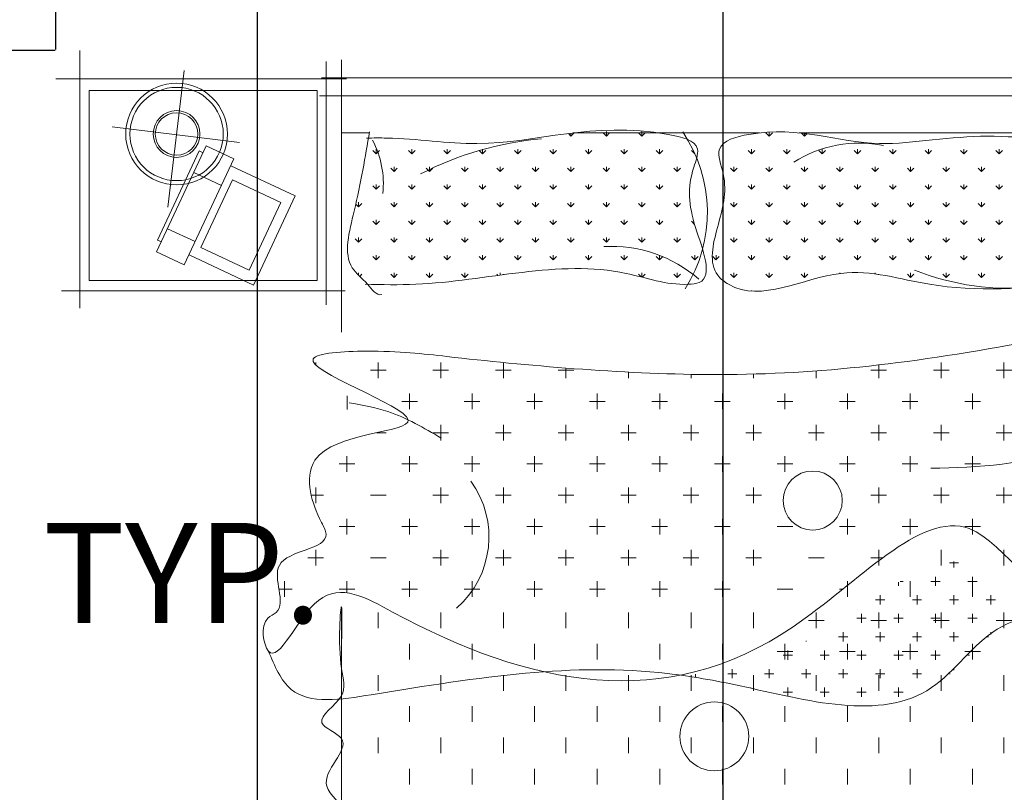
# Model space of a CAD drawing. Units: inches. Extents: x -438 to 102, y -60 to 1091.
# Tile 12 of 20: x -322 to -243, y 961 to 1022. Entities that reach past the tile are written whole.
import ezdxf

# ---------------------------------------------------------------- set-up
doc = ezdxf.new("R2010")
doc.units = ezdxf.units.IN
doc.header["$MEASUREMENT"] = 0
doc.layers.add('A-ANNO-DIMS', color=217, linetype='Continuous', lineweight=18, true_color=0x93278f)
doc.layers.add('Furniture', color=7, linetype='Continuous', lineweight=15)
doc.styles.get("Standard").update_dxf_attribs({"font": 'arial.ttf'})
doc.dimstyles.get("Standard").update_dxf_attribs({"dimtxt": 8, "dimasz": 0.18, "dimexe": 0.18, "dimexo": 0.0625, "dimgap": 0.09, "dimtad": 0, "dimtih": 1, "dimtoh": 1, "dimdec": 4, "dimzin": 0, "dimdsep": 46, "dimlunit": 3, "dimtxsty": 'Standard', "dimcen": 0.09, "dimadec": 0, "dimazin": 0, "dimtfac": 1, "dimtdec": 4, "dimtofl": 0, "dimtmove": 0, "dimatfit": 3, "dimfxl": 1, "dimtolj": 1, "dimtzin": 0, "dimarcsym": 0})

# ---------------------------------------------------------------- blocks, each defined once
blk = doc.blocks.new('BED-DOUBLE-WITH-NIGHTSTANDS')
for p, q in [((-50.059, 0.003), (-50.059, -20.597)), ((-29.157, -22.53), (-29.157, -0.743)), ((-30.374, -20.327), (-30.374, -0.897)), ((-28.759, -2.28), (-51.984, -2.28)), ((-41.716, -1.597), (-43.046, -12.532)), ((-30.745, -2.188), (29.898, -2.188)), ((-31.095, -3.205), (-49.317, -3.205)), ((-49.317, -3.205), (-49.317, -18.39)), ((-31.095, -18.39), (-31.095, -3.205)), ((30.685, -3.641), (-30.922, -3.641)), ((-37.317, -7.352), (-47.474, -6.101)), ((-26.928, -6.593), (-29.157, -6.593)), ((-10.816, -6.85), (-11.024, -6.642)), ((-10.816, -6.85), (-10.551, -6.585)), ((-10.816, -6.851), (-10.816, -6.616)), ((4.241, -6.593), (-10.627, -6.593)), ((-7.988, -6.85), (-8.253, -6.585)), ((-7.988, -6.85), (-7.723, -6.585)), ((-7.987, -6.851), (-7.987, -6.476)), ((-5.159, -6.85), (-5.425, -6.585)), ((-5.159, -6.851), (-5.159, -6.476)), ((-5.159, -6.85), (-4.894, -6.585)), ((5.018, -6.85), (4.753, -6.585)), ((5.018, -6.851), (5.018, -6.53)), ((5.018, -6.85), (5.283, -6.585)), ((29.898, -6.593), (7.41, -6.593)), ((7.846, -6.85), (7.61, -6.614)), ((7.846, -6.85), (8.033, -6.663)), ((7.847, -6.851), (7.847, -6.641)), ((-43.928, -16.114), (-39.959, -7.633)), ((-39.959, -7.633), (-37.75, -8.667)), ((-40.527, -8.034), (-43.863, -15.161)), ((-40.215, -8.18), (-40.527, -8.034)), ((-26.373, -8.265), (-26.638, -8)), ((-26.373, -8.265), (-26.107, -8)), ((-26.372, -8.265), (-26.372, -7.89)), ((-23.544, -8.265), (-23.809, -8)), ((-23.544, -8.265), (-23.544, -7.89)), ((-23.544, -8.265), (-23.279, -8)), ((-20.716, -8.265), (-20.981, -8)), ((-20.716, -8.265), (-20.451, -8)), ((-20.715, -8.265), (-20.715, -7.89)), ((-17.887, -8.265), (-18.152, -8)), ((-17.887, -8.265), (-17.887, -7.89)), ((-17.887, -8.265), (-17.622, -8)), ((-15.059, -8.265), (-15.324, -8)), ((-15.059, -8.265), (-14.794, -8)), ((-15.058, -8.265), (-15.058, -7.89)), ((-12.23, -8.265), (-12.496, -8)), ((-12.23, -8.265), (-12.23, -7.89)), ((-12.23, -8.265), (-11.965, -8)), ((-9.402, -8.265), (-9.667, -8)), ((-9.402, -8.265), (-9.402, -7.89)), ((-9.402, -8.265), (-9.137, -8)), ((-6.574, -8.265), (-6.839, -8)), ((-6.574, -8.265), (-6.308, -8)), ((-6.573, -8.265), (-6.573, -7.89)), ((-3.745, -8.265), (-4.01, -8)), ((-3.745, -8.265), (-3.745, -7.89)), ((-3.745, -8.265), (-3.48, -8)), ((-0.917, -8.265), (-1.182, -8)), ((-0.917, -8.265), (-0.915, -8.262)), ((-0.916, -8.265), (-0.916, -8.258)), ((1.02, -8.021), (1.041, -8)), ((3.604, -8.265), (3.339, -8)), ((3.604, -8.265), (3.604, -7.89)), ((3.604, -8.265), (3.869, -8)), ((6.432, -8.265), (6.167, -8)), ((6.432, -8.265), (6.697, -8)), ((6.433, -8.265), (6.433, -7.89)), ((9.261, -8.265), (8.996, -8)), ((9.261, -8.265), (9.261, -7.89)), ((9.261, -8.265), (9.526, -8)), ((12.089, -8.265), (11.824, -8)), ((12.089, -8.265), (12.089, -7.89)), ((12.089, -8.265), (12.354, -8)), ((14.918, -8.265), (14.652, -8)), ((14.918, -8.265), (14.918, -7.89)), ((14.918, -8.265), (15.183, -8)), ((17.746, -8.265), (17.481, -8)), ((17.746, -8.265), (17.746, -7.89)), ((17.746, -8.265), (18.011, -8)), ((20.574, -8.265), (20.309, -8)), ((20.574, -8.265), (20.84, -8)), ((20.575, -8.265), (20.575, -7.89)), ((23.403, -8.265), (23.138, -8)), ((23.403, -8.265), (23.403, -7.89)), ((23.403, -8.265), (23.668, -8)), ((-37.75, -8.667), (-41.72, -17.147)), ((-32.845, -11.63), (-38.006, -9.214)), ((-24.958, -9.679), (-25.224, -9.414)), ((-24.958, -9.679), (-24.958, -9.304)), ((-24.958, -9.679), (-24.693, -9.414)), ((-22.13, -9.679), (-22.395, -9.414)), ((-22.13, -9.679), (-22.13, -9.304)), ((-22.13, -9.679), (-21.865, -9.414)), ((-19.302, -9.679), (-19.567, -9.414)), ((-19.302, -9.679), (-19.036, -9.414)), ((-19.301, -9.679), (-19.301, -9.304)), ((-16.473, -9.679), (-16.738, -9.414)), ((-16.473, -9.679), (-16.473, -9.304)), ((-16.473, -9.679), (-16.208, -9.414)), ((-13.645, -9.679), (-13.91, -9.414)), ((-13.645, -9.679), (-13.38, -9.414)), ((-13.644, -9.679), (-13.644, -9.304)), ((-10.816, -9.679), (-11.081, -9.414)), ((-10.816, -9.679), (-10.816, -9.304)), ((-10.816, -9.679), (-10.551, -9.414)), ((-7.988, -9.679), (-8.253, -9.414)), ((-7.988, -9.679), (-7.723, -9.414)), ((-7.987, -9.679), (-7.987, -9.304)), ((-5.159, -9.679), (-5.425, -9.414)), ((-5.159, -9.679), (-5.159, -9.304)), ((-5.159, -9.679), (-4.894, -9.414)), ((-2.331, -9.679), (-2.596, -9.414)), ((-2.331, -9.679), (-2.331, -9.304)), ((-2.331, -9.679), (-2.066, -9.414)), ((2.19, -9.679), (1.924, -9.414)), ((2.19, -9.679), (2.19, -9.304)), ((2.19, -9.679), (2.455, -9.414)), ((5.018, -9.679), (4.753, -9.414)), ((5.018, -9.679), (5.018, -9.304)), ((5.018, -9.679), (5.283, -9.414)), ((7.846, -9.679), (7.581, -9.414)), ((7.846, -9.679), (8.112, -9.414)), ((7.847, -9.679), (7.847, -9.304)), ((10.675, -9.679), (10.41, -9.414)), ((10.675, -9.679), (10.675, -9.304)), ((10.675, -9.679), (10.94, -9.414)), ((13.503, -9.679), (13.238, -9.414)), ((13.503, -9.679), (13.768, -9.414)), ((13.504, -9.679), (13.504, -9.304)), ((16.332, -9.679), (16.067, -9.414)), ((16.332, -9.679), (16.332, -9.304)), ((16.332, -9.679), (16.597, -9.414)), ((19.16, -9.679), (18.895, -9.414)), ((19.16, -9.679), (19.425, -9.414)), ((19.161, -9.679), (19.161, -9.304)), ((21.989, -9.679), (21.723, -9.414)), ((21.989, -9.679), (21.989, -9.304)), ((21.989, -9.679), (22.254, -9.414)), ((-38.742, -10.787), (-40.951, -9.753)), ((-37.855, -10.358), (-40.387, -15.767)), ((-34.001, -12.162), (-37.855, -10.358)), ((-26.373, -11.093), (-26.638, -10.828)), ((-26.373, -11.093), (-26.107, -10.828)), ((-26.372, -11.093), (-26.372, -10.718)), ((-23.544, -11.093), (-23.809, -10.828)), ((-23.544, -11.093), (-23.544, -10.718)), ((-23.544, -11.093), (-23.279, -10.828)), ((-20.716, -11.093), (-20.981, -10.828)), ((-20.716, -11.093), (-20.451, -10.828)), ((-20.715, -11.093), (-20.715, -10.718)), ((-17.887, -11.093), (-18.152, -10.828)), ((-17.887, -11.093), (-17.887, -10.718)), ((-17.887, -11.093), (-17.622, -10.828)), ((-15.059, -11.093), (-15.324, -10.828)), ((-15.059, -11.093), (-14.794, -10.828)), ((-15.058, -11.093), (-15.058, -10.718)), ((-12.23, -11.093), (-12.496, -10.828)), ((-12.23, -11.093), (-12.23, -10.718)), ((-12.23, -11.093), (-11.965, -10.828)), ((-9.402, -11.093), (-9.667, -10.828)), ((-9.402, -11.093), (-9.402, -10.718)), ((-9.402, -11.093), (-9.137, -10.828)), ((-6.574, -11.093), (-6.839, -10.828)), ((-6.574, -11.093), (-6.308, -10.828)), ((-6.573, -11.093), (-6.573, -10.718)), ((-3.745, -11.093), (-4.01, -10.828)), ((-3.745, -11.093), (-3.745, -10.718)), ((-3.745, -11.093), (-3.48, -10.828)), ((3.604, -11.093), (3.339, -10.828)), ((3.604, -11.093), (3.604, -10.718)), ((3.604, -11.093), (3.869, -10.828)), ((6.432, -11.093), (6.167, -10.828)), ((6.432, -11.093), (6.697, -10.828)), ((6.433, -11.093), (6.433, -10.718)), ((9.261, -11.093), (8.996, -10.828)), ((9.261, -11.093), (9.261, -10.718)), ((9.261, -11.093), (9.526, -10.828)), ((12.089, -11.093), (11.824, -10.828)), ((12.089, -11.093), (12.089, -10.718)), ((12.089, -11.093), (12.354, -10.828)), ((14.918, -11.093), (14.652, -10.828)), ((14.918, -11.093), (14.918, -10.718)), ((14.918, -11.093), (15.183, -10.828)), ((17.746, -11.093), (17.481, -10.828)), ((17.746, -11.093), (17.746, -10.718)), ((17.746, -11.093), (18.011, -10.828)), ((20.574, -11.093), (20.309, -10.828)), ((20.574, -11.093), (20.84, -10.828)), ((20.575, -11.093), (20.575, -10.718)), ((23.403, -11.093), (23.138, -10.828)), ((23.403, -11.093), (23.403, -10.718)), ((23.403, -11.093), (23.668, -10.828)), ((-36.181, -18.757), (-32.845, -11.63)), ((-36.532, -17.571), (-34.001, -12.162)), ((-27.787, -12.507), (-28.013, -12.281)), ((-27.787, -12.507), (-27.522, -12.242)), ((-27.786, -12.508), (-27.786, -12.133)), ((-24.958, -12.507), (-25.224, -12.242)), ((-24.958, -12.508), (-24.958, -12.133)), ((-24.958, -12.507), (-24.693, -12.242)), ((-22.13, -12.507), (-22.395, -12.242)), ((-22.13, -12.508), (-22.13, -12.133)), ((-22.13, -12.507), (-21.865, -12.242)), ((-19.302, -12.507), (-19.567, -12.242)), ((-19.302, -12.507), (-19.036, -12.242)), ((-19.301, -12.508), (-19.301, -12.133)), ((-16.473, -12.507), (-16.738, -12.242)), ((-16.473, -12.508), (-16.473, -12.133)), ((-16.473, -12.507), (-16.208, -12.242)), ((-13.645, -12.507), (-13.91, -12.242)), ((-13.645, -12.507), (-13.38, -12.242)), ((-13.644, -12.508), (-13.644, -12.133)), ((-10.816, -12.507), (-11.081, -12.242)), ((-10.816, -12.508), (-10.816, -12.133)), ((-10.816, -12.507), (-10.551, -12.242)), ((-7.988, -12.507), (-8.253, -12.242)), ((-7.988, -12.507), (-7.723, -12.242)), ((-7.987, -12.508), (-7.987, -12.133)), ((-5.159, -12.507), (-5.425, -12.242)), ((-5.159, -12.508), (-5.159, -12.133)), ((-5.159, -12.507), (-4.894, -12.242)), ((-2.331, -12.507), (-2.596, -12.242)), ((-2.331, -12.508), (-2.331, -12.133)), ((-2.331, -12.507), (-2.066, -12.242)), ((2.19, -12.507), (1.924, -12.242)), ((2.19, -12.508), (2.19, -12.133)), ((2.19, -12.507), (2.455, -12.242)), ((5.018, -12.507), (4.753, -12.242)), ((5.018, -12.508), (5.018, -12.133)), ((5.018, -12.507), (5.283, -12.242)), ((7.846, -12.507), (7.581, -12.242)), ((7.846, -12.507), (8.112, -12.242)), ((7.847, -12.508), (7.847, -12.133)), ((10.675, -12.507), (10.41, -12.242)), ((10.675, -12.508), (10.675, -12.133)), ((10.675, -12.507), (10.94, -12.242)), ((13.503, -12.507), (13.238, -12.242)), ((13.503, -12.507), (13.768, -12.242)), ((13.504, -12.508), (13.504, -12.133)), ((16.332, -12.507), (16.067, -12.242)), ((16.332, -12.508), (16.332, -12.133)), ((16.332, -12.507), (16.597, -12.242)), ((19.16, -12.507), (18.895, -12.242)), ((19.16, -12.507), (19.425, -12.242)), ((19.161, -12.508), (19.161, -12.133)), ((21.989, -12.507), (21.723, -12.242)), ((21.989, -12.508), (21.989, -12.133)), ((21.989, -12.507), (22.254, -12.242)), ((-26.373, -13.922), (-26.638, -13.656)), ((-26.373, -13.922), (-26.107, -13.656)), ((-26.372, -13.922), (-26.372, -13.547)), ((-23.544, -13.922), (-23.809, -13.656)), ((-23.544, -13.922), (-23.544, -13.547)), ((-23.544, -13.922), (-23.279, -13.656)), ((-20.716, -13.922), (-20.981, -13.656)), ((-20.716, -13.922), (-20.451, -13.656)), ((-20.715, -13.922), (-20.715, -13.547)), ((-17.887, -13.922), (-18.152, -13.656)), ((-17.887, -13.922), (-17.887, -13.547)), ((-17.887, -13.922), (-17.622, -13.656)), ((-15.059, -13.922), (-15.324, -13.656)), ((-15.059, -13.922), (-14.794, -13.656)), ((-15.058, -13.922), (-15.058, -13.547)), ((-12.23, -13.922), (-12.496, -13.656)), ((-12.23, -13.922), (-12.23, -13.547)), ((-12.23, -13.922), (-11.965, -13.656)), ((-9.402, -13.922), (-9.667, -13.656)), ((-9.402, -13.922), (-9.402, -13.547)), ((-9.402, -13.922), (-9.137, -13.656)), ((-6.574, -13.922), (-6.839, -13.656)), ((-6.574, -13.922), (-6.308, -13.656)), ((-6.573, -13.922), (-6.573, -13.547)), ((-3.745, -13.922), (-4.01, -13.656)), ((-3.745, -13.922), (-3.745, -13.547)), ((-3.745, -13.922), (-3.48, -13.656)), ((-0.933, -13.906), (-1.182, -13.656)), ((1.022, -13.675), (1.041, -13.656)), ((3.604, -13.922), (3.339, -13.656)), ((3.604, -13.922), (3.604, -13.547)), ((3.604, -13.922), (3.869, -13.656)), ((6.432, -13.922), (6.167, -13.656)), ((6.432, -13.922), (6.697, -13.656)), ((6.433, -13.922), (6.433, -13.547)), ((9.261, -13.922), (8.996, -13.656)), ((9.261, -13.922), (9.261, -13.547)), ((9.261, -13.922), (9.526, -13.656)), ((12.089, -13.922), (11.824, -13.656)), ((12.089, -13.922), (12.089, -13.547)), ((12.089, -13.922), (12.354, -13.656)), ((14.918, -13.922), (14.652, -13.656)), ((14.918, -13.922), (14.918, -13.547)), ((14.918, -13.922), (15.183, -13.656)), ((17.746, -13.922), (17.481, -13.656)), ((17.746, -13.922), (17.746, -13.547)), ((17.746, -13.922), (18.011, -13.656)), ((20.574, -13.922), (20.309, -13.656)), ((20.574, -13.922), (20.84, -13.656)), ((20.575, -13.922), (20.575, -13.547)), ((23.403, -13.922), (23.138, -13.656)), ((23.403, -13.922), (23.403, -13.547)), ((23.403, -13.922), (23.668, -13.656)), ((-40.849, -15.287), (-43.058, -14.253)), ((-43.863, -15.161), (-43.551, -15.307)), ((-27.787, -15.336), (-28.052, -15.071)), ((-27.787, -15.336), (-27.522, -15.071)), ((-27.786, -15.336), (-27.786, -14.961)), ((-24.958, -15.336), (-25.224, -15.071)), ((-24.958, -15.336), (-24.958, -14.961)), ((-24.958, -15.336), (-24.693, -15.071)), ((-22.13, -15.336), (-22.395, -15.071)), ((-22.13, -15.336), (-22.13, -14.961)), ((-22.13, -15.336), (-21.865, -15.071)), ((-19.302, -15.336), (-19.567, -15.071)), ((-19.302, -15.336), (-19.036, -15.071)), ((-19.301, -15.336), (-19.301, -14.961)), ((-16.473, -15.336), (-16.738, -15.071)), ((-16.473, -15.336), (-16.473, -14.961)), ((-16.473, -15.336), (-16.208, -15.071)), ((-13.645, -15.336), (-13.91, -15.071)), ((-13.645, -15.336), (-13.38, -15.071)), ((-13.644, -15.336), (-13.644, -14.961)), ((-10.816, -15.336), (-11.081, -15.071)), ((-10.816, -15.336), (-10.816, -14.961)), ((-10.816, -15.336), (-10.551, -15.071)), ((-7.988, -15.336), (-8.253, -15.071)), ((-7.988, -15.336), (-7.723, -15.071)), ((-7.987, -15.336), (-7.987, -14.961)), ((-5.159, -15.336), (-5.425, -15.071)), ((-5.159, -15.336), (-5.159, -14.961)), ((-5.159, -15.336), (-4.894, -15.071)), ((-2.331, -15.336), (-2.596, -15.071)), ((-2.331, -15.336), (-2.331, -14.961)), ((-2.331, -15.336), (-2.066, -15.071)), ((2.19, -15.336), (1.924, -15.071)), ((2.19, -15.336), (2.19, -14.961)), ((2.19, -15.336), (2.455, -15.071)), ((5.018, -15.336), (4.753, -15.071)), ((5.018, -15.336), (5.018, -14.961)), ((5.018, -15.336), (5.283, -15.071)), ((7.846, -15.336), (7.581, -15.071)), ((7.846, -15.336), (8.112, -15.071)), ((7.847, -15.336), (7.847, -14.961)), ((10.675, -15.336), (10.41, -15.071)), ((10.675, -15.336), (10.675, -14.961)), ((10.675, -15.336), (10.94, -15.071)), ((13.503, -15.336), (13.238, -15.071)), ((13.503, -15.336), (13.768, -15.071)), ((13.504, -15.336), (13.504, -14.961)), ((16.332, -15.336), (16.067, -15.071)), ((16.332, -15.336), (16.332, -14.961)), ((16.332, -15.336), (16.597, -15.071)), ((19.16, -15.336), (18.895, -15.071)), ((19.16, -15.336), (19.425, -15.071)), ((19.161, -15.336), (19.161, -14.961)), ((21.989, -15.336), (21.723, -15.071)), ((21.989, -15.336), (21.989, -14.961)), ((21.989, -15.336), (22.254, -15.071)), ((-41.72, -17.147), (-43.928, -16.114)), ((-41.342, -16.341), (-36.181, -18.757)), ((-40.387, -15.767), (-36.532, -17.571)), ((-26.373, -16.75), (-26.638, -16.485)), ((-26.373, -16.75), (-26.107, -16.485)), ((-26.372, -16.75), (-26.372, -16.375)), ((-23.544, -16.75), (-23.809, -16.485)), ((-23.544, -16.75), (-23.544, -16.375)), ((-23.544, -16.75), (-23.279, -16.485)), ((-20.716, -16.75), (-20.981, -16.485)), ((-20.716, -16.75), (-20.451, -16.485)), ((-20.715, -16.75), (-20.715, -16.375)), ((-17.887, -16.75), (-18.152, -16.485)), ((-17.887, -16.75), (-17.887, -16.375)), ((-17.887, -16.75), (-17.622, -16.485)), ((-15.059, -16.75), (-15.324, -16.485)), ((-15.059, -16.75), (-14.794, -16.485)), ((-15.058, -16.75), (-15.058, -16.375)), ((-12.23, -16.75), (-12.496, -16.485)), ((-12.23, -16.75), (-12.23, -16.375)), ((-12.23, -16.75), (-11.965, -16.485)), ((-9.402, -16.75), (-9.667, -16.485)), ((-9.402, -16.75), (-9.402, -16.375)), ((-9.402, -16.75), (-9.137, -16.485)), ((-6.574, -16.75), (-6.839, -16.485)), ((-6.574, -16.75), (-6.308, -16.485)), ((-6.573, -16.75), (-6.573, -16.375)), ((-3.745, -16.75), (-4.01, -16.485)), ((-3.745, -16.75), (-3.745, -16.375)), ((-3.745, -16.75), (-3.48, -16.485)), ((-0.917, -16.75), (-1.182, -16.485)), ((-0.917, -16.75), (-0.652, -16.485)), ((-0.916, -16.75), (-0.916, -16.375)), ((0.775, -16.75), (0.51, -16.485)), ((0.775, -16.75), (1.041, -16.485)), ((0.776, -16.75), (0.776, -16.375)), ((3.604, -16.75), (3.339, -16.485)), ((3.604, -16.75), (3.604, -16.375)), ((3.604, -16.75), (3.869, -16.485)), ((6.432, -16.75), (6.167, -16.485)), ((6.432, -16.75), (6.697, -16.485)), ((6.433, -16.75), (6.433, -16.375)), ((9.261, -16.75), (8.996, -16.485)), ((9.261, -16.75), (9.261, -16.375)), ((9.261, -16.75), (9.526, -16.485)), ((12.089, -16.75), (11.824, -16.485)), ((12.089, -16.75), (12.089, -16.375)), ((12.089, -16.75), (12.354, -16.485)), ((14.918, -16.75), (14.652, -16.485)), ((14.918, -16.75), (14.918, -16.375)), ((14.918, -16.75), (15.183, -16.485)), ((17.746, -16.75), (17.481, -16.485)), ((17.746, -16.75), (17.746, -16.375)), ((17.746, -16.75), (18.011, -16.485)), ((20.574, -16.75), (20.309, -16.485)), ((20.574, -16.75), (20.84, -16.485)), ((20.575, -16.75), (20.575, -16.375)), ((23.403, -16.75), (23.138, -16.485)), ((23.403, -16.75), (23.403, -16.375)), ((23.403, -16.75), (23.668, -16.485)), ((-27.786, -17.973), (-27.786, -17.79)), ((-27.69, -18.067), (-27.522, -17.899)), ((-24.958, -18.164), (-25.224, -17.899)), ((-24.958, -18.165), (-24.958, -17.79)), ((-24.958, -18.164), (-24.693, -17.899)), ((-22.13, -18.164), (-22.395, -17.899)), ((-22.13, -18.165), (-22.13, -17.79)), ((-22.13, -18.164), (-21.865, -17.899)), ((-19.302, -18.164), (-19.567, -17.899)), ((-19.302, -18.164), (-19.036, -17.899)), ((-19.301, -18.165), (-19.301, -17.79)), ((-16.65, -17.987), (-16.738, -17.899)), ((-16.473, -17.964), (-16.473, -17.79)), ((-16.242, -17.933), (-16.208, -17.899)), ((-5.211, -18.113), (-5.425, -17.899)), ((-5.159, -18.126), (-5.159, -17.79)), ((-5.129, -18.134), (-4.894, -17.899)), ((-2.331, -18.164), (-2.596, -17.899)), ((-2.331, -18.165), (-2.331, -17.79)), ((-2.331, -18.164), (-2.066, -17.899)), ((2.19, -18.164), (1.924, -17.899)), ((2.19, -18.165), (2.19, -17.79)), ((2.19, -18.164), (2.455, -17.899)), ((5.018, -18.164), (4.753, -17.899)), ((5.018, -18.165), (5.018, -17.79)), ((5.018, -18.164), (5.283, -17.899)), ((7.846, -18.164), (7.581, -17.899)), ((7.846, -18.164), (8.112, -17.899)), ((7.847, -18.165), (7.847, -17.79)), ((10.675, -17.833), (10.675, -17.79)), ((13.504, -17.877), (13.504, -17.79)), ((13.756, -17.912), (13.768, -17.899)), ((16.332, -18.164), (16.067, -17.899)), ((16.332, -18.165), (16.332, -17.79)), ((16.332, -18.164), (16.597, -17.899)), ((19.16, -18.164), (18.895, -17.899)), ((19.16, -18.164), (19.425, -17.899)), ((19.161, -18.165), (19.161, -17.79)), ((21.989, -18.164), (21.723, -17.899)), ((21.989, -18.165), (21.989, -17.79)), ((21.989, -18.164), (22.254, -17.899)), ((-49.317, -18.39), (-31.095, -18.39)), ((-51.534, -19.209), (-28.849, -19.209)), ((3.604, -19.237), (3.604, -19.204)), ((-31.218, -25.145), (-31.218, -24.94)), ((-26.218, -26.19), (-26.218, -24.94)), ((-21.218, -26.19), (-21.218, -24.94)), ((-16.218, -26.19), (-16.218, -24.951)), ((13.782, -26.19), (13.782, -25.145)), ((18.782, -26.19), (18.782, -24.94)), ((23.782, -26.19), (23.782, -24.94)), ((-30.593, -25.565), (-30.673, -25.565)), ((-25.593, -25.565), (-26.843, -25.565)), ((-20.593, -25.565), (-21.843, -25.565)), ((-15.593, -25.565), (-16.843, -25.565)), ((-10.593, -25.565), (-11.843, -25.565)), ((-11.218, -26.19), (-11.218, -25.392)), ((-6.218, -26.19), (-6.218, -25.718)), ((-1.218, -26.19), (-1.218, -25.896)), ((3.782, -26.19), (3.782, -25.874)), ((8.782, -26.19), (8.782, -25.623)), ((14.407, -25.565), (13.157, -25.565)), ((19.407, -25.565), (18.157, -25.565)), ((24.407, -25.565), (23.157, -25.565)), ((-23.718, -28.69), (-23.718, -27.44)), ((-18.718, -28.69), (-18.718, -27.44)), ((-13.718, -28.69), (-13.718, -27.44)), ((-8.718, -28.69), (-8.718, -27.44)), ((-3.718, -28.69), (-3.718, -27.44)), ((1.282, -28.69), (1.282, -27.44)), ((6.282, -28.69), (6.282, -27.44)), ((11.282, -28.69), (11.282, -27.44)), ((16.282, -28.69), (16.282, -27.44)), ((21.282, -28.69), (21.282, -27.44)), ((-28.711, -28.721), (-28.711, -27.603)), ((-23.093, -28.065), (-24.343, -28.065)), ((-18.093, -28.065), (-19.343, -28.065)), ((-13.093, -28.065), (-14.343, -28.065)), ((-8.093, -28.065), (-9.343, -28.065)), ((-3.093, -28.065), (-4.343, -28.065)), ((1.907, -28.065), (0.657, -28.065)), ((6.907, -28.065), (5.657, -28.065)), ((11.907, -28.065), (10.657, -28.065)), ((16.907, -28.065), (15.657, -28.065)), ((21.907, -28.065), (20.657, -28.065)), ((-25.593, -30.565), (-26.366, -30.565)), ((-20.593, -30.565), (-21.843, -30.565)), ((-21.218, -31.19), (-21.218, -29.94)), ((-15.593, -30.565), (-16.843, -30.565)), ((-16.218, -31.19), (-16.218, -29.94)), ((-10.593, -30.565), (-11.843, -30.565)), ((-11.218, -31.19), (-11.218, -29.94)), ((-5.593, -30.565), (-6.843, -30.565)), ((-6.218, -31.19), (-6.218, -29.94)), ((-0.593, -30.565), (-1.843, -30.565)), ((-1.218, -31.19), (-1.218, -29.94)), ((4.407, -30.565), (3.157, -30.565)), ((3.782, -31.19), (3.782, -29.94)), ((9.407, -30.565), (8.157, -30.565)), ((8.782, -31.19), (8.782, -29.94)), ((14.407, -30.565), (13.157, -30.565)), ((13.782, -31.19), (13.782, -29.94)), ((19.407, -30.565), (18.157, -30.565)), ((18.782, -31.19), (18.782, -29.94)), ((24.407, -30.565), (23.157, -30.565)), ((23.782, -31.19), (23.782, -29.94)), ((-28.718, -33.69), (-28.718, -32.44)), ((-23.718, -33.69), (-23.718, -32.44)), ((-18.718, -33.69), (-18.718, -32.44)), ((-13.718, -33.69), (-13.718, -32.44)), ((-8.718, -33.69), (-8.718, -32.44)), ((-3.718, -33.69), (-3.718, -32.44)), ((1.282, -33.69), (1.282, -32.44)), ((6.282, -33.69), (6.282, -32.44)), ((11.282, -33.69), (11.282, -32.44)), ((16.282, -33.69), (16.282, -32.44)), ((21.282, -33.69), (21.282, -32.44)), ((-28.093, -33.065), (-29.343, -33.065)), ((-23.093, -33.065), (-24.343, -33.065)), ((-18.093, -33.065), (-19.343, -33.065)), ((-13.093, -33.065), (-14.343, -33.065)), ((-8.093, -33.065), (-9.343, -33.065)), ((-3.093, -33.065), (-4.343, -33.065)), ((1.907, -33.065), (0.657, -33.065)), ((6.907, -33.065), (5.657, -33.065)), ((11.907, -33.065), (10.657, -33.065)), ((16.907, -33.065), (15.657, -33.065)), ((21.907, -33.065), (20.657, -33.065)), ((-31.218, -36.19), (-31.218, -34.94)), ((-21.218, -36.19), (-21.218, -34.94)), ((-16.218, -36.19), (-16.218, -34.94)), ((-11.218, -36.19), (-11.218, -34.94)), ((-6.218, -36.19), (-6.218, -34.94)), ((-1.218, -36.19), (-1.218, -34.94)), ((3.782, -36.19), (3.782, -34.94)), ((13.782, -36.19), (13.782, -34.94)), ((18.782, -36.19), (18.782, -34.94)), ((23.782, -36.19), (23.782, -34.94)), ((-30.593, -35.565), (-31.573, -35.565)), ((-25.593, -35.565), (-26.843, -35.565)), ((-20.593, -35.565), (-21.843, -35.565)), ((-15.593, -35.565), (-16.843, -35.565)), ((-10.593, -35.565), (-11.843, -35.565)), ((-5.593, -35.565), (-6.843, -35.565)), ((-0.593, -35.565), (-1.843, -35.565)), ((4.407, -35.565), (3.157, -35.565)), ((14.407, -35.565), (13.157, -35.565)), ((19.407, -35.565), (18.157, -35.565)), ((24.407, -35.565), (23.157, -35.565)), ((-28.718, -38.69), (-28.718, -37.44)), ((-23.718, -38.69), (-23.718, -37.44)), ((-18.718, -38.69), (-18.718, -37.44)), ((-13.718, -38.69), (-13.718, -37.44)), ((-8.718, -38.69), (-8.718, -37.44)), ((-3.718, -38.69), (-3.718, -37.44)), ((1.282, -38.69), (1.282, -37.44)), ((11.282, -38.69), (11.282, -37.44)), ((16.282, -38.69), (16.282, -37.44)), ((21.282, -38.69), (21.282, -37.44)), ((-28.093, -38.065), (-29.343, -38.065)), ((-23.093, -38.065), (-24.343, -38.065)), ((-18.093, -38.065), (-19.343, -38.065)), ((-13.093, -38.065), (-14.343, -38.065)), ((-8.093, -38.065), (-9.343, -38.065)), ((-3.093, -38.065), (-4.343, -38.065)), ((1.907, -38.065), (0.657, -38.065)), ((6.907, -38.065), (5.657, -38.065)), ((11.907, -38.065), (10.657, -38.065)), ((16.907, -38.065), (15.657, -38.065)), ((21.907, -38.065), (20.657, -38.065)), ((-31.218, -41.19), (-31.218, -39.94)), ((-21.218, -41.19), (-21.218, -39.94)), ((-16.218, -41.19), (-16.218, -39.94)), ((-11.218, -41.19), (-11.218, -39.94)), ((-6.218, -41.19), (-6.218, -39.94)), ((-1.218, -41.19), (-1.218, -39.94)), ((3.782, -41.19), (3.782, -39.94)), ((13.782, -41.19), (13.782, -39.94)), ((18.782, -41.19), (18.782, -39.94)), ((23.782, -41.19), (23.782, -39.94)), ((-30.593, -40.565), (-31.843, -40.565)), ((-25.593, -40.565), (-26.843, -40.565)), ((-20.593, -40.565), (-21.843, -40.565)), ((-15.593, -40.565), (-16.843, -40.565)), ((-10.593, -40.565), (-11.843, -40.565)), ((-5.593, -40.565), (-6.843, -40.565)), ((-0.593, -40.565), (-1.843, -40.565)), ((4.407, -40.565), (3.157, -40.565)), ((9.407, -40.565), (8.157, -40.565)), ((14.104, -40.565), (13.157, -40.565)), ((19.795, -41.341), (19.795, -40.863)), ((20.164, -40.972), (19.426, -40.972)), ((-33.718, -43.69), (-33.718, -42.44)), ((-28.718, -43.367), (-28.718, -42.44)), ((-23.718, -43.69), (-23.718, -42.44)), ((-18.718, -43.69), (-18.718, -42.44)), ((-13.718, -43.69), (-13.718, -42.44)), ((-8.718, -43.69), (-8.718, -42.44)), ((-3.718, -43.69), (-3.718, -42.44)), ((1.282, -43.69), (1.282, -42.44)), ((11.282, -43.69), (11.282, -42.44)), ((15.735, -42.448), (15.495, -42.448)), ((16.282, -43.69), (16.282, -42.44)), ((18.688, -42.448), (17.949, -42.448)), ((18.318, -42.817), (18.318, -42.079)), ((21.64, -42.448), (20.902, -42.448)), ((21.271, -42.817), (21.271, -42.079)), ((21.282, -43.69), (21.282, -42.44)), ((-33.093, -43.065), (-34.154, -43.065)), ((-28.093, -43.065), (-29.343, -43.065)), ((-23.093, -43.065), (-24.343, -43.065)), ((-18.093, -43.065), (-19.343, -43.065)), ((-13.093, -43.065), (-14.343, -43.065)), ((-8.093, -43.065), (-9.343, -43.065)), ((-3.093, -43.065), (-4.343, -43.065)), ((1.907, -43.065), (0.657, -43.065)), ((6.907, -43.065), (5.657, -43.065)), ((10.916, -43.065), (10.657, -43.065)), ((15.366, -42.817), (15.366, -42.522)), ((14.258, -43.924), (13.52, -43.924)), ((13.889, -44.294), (13.889, -43.555)), ((17.211, -43.924), (16.473, -43.924)), ((16.842, -44.294), (16.842, -43.555)), ((20.164, -43.924), (19.426, -43.924)), ((19.795, -44.294), (19.795, -43.555)), ((23.117, -43.924), (22.378, -43.924)), ((22.748, -44.294), (22.748, -43.555)), ((-29.157, -79.94), (-29.157, -44.493)), ((-26.218, -46.19), (-26.218, -44.94)), ((-21.218, -46.19), (-21.218, -44.94)), ((-16.218, -46.19), (-16.218, -44.94)), ((-11.218, -46.19), (-11.218, -44.94)), ((-6.218, -46.19), (-6.218, -44.94)), ((-1.218, -46.19), (-1.218, -44.94)), ((3.782, -46.19), (3.782, -44.94)), ((9.407, -45.565), (8.157, -45.565)), ((8.782, -46.19), (8.782, -44.94)), ((12.782, -45.401), (12.044, -45.401)), ((12.413, -45.77), (12.413, -45.032)), ((14.407, -45.565), (13.157, -45.565)), ((13.782, -46.19), (13.782, -44.94)), ((15.735, -45.401), (14.997, -45.401)), ((15.366, -45.77), (15.366, -45.032)), ((18.688, -45.401), (17.949, -45.401)), ((19.407, -45.565), (18.157, -45.565)), ((18.318, -45.77), (18.318, -45.032)), ((18.782, -46.19), (18.782, -44.94)), ((21.64, -45.401), (20.902, -45.401)), ((21.271, -45.77), (21.271, -45.032)), ((24.407, -45.565), (23.157, -45.565)), ((23.782, -46.19), (23.782, -44.94)), ((7.984, -47.246), (7.984, -47.199)), ((11.306, -46.877), (10.567, -46.877)), ((10.937, -47.246), (10.937, -46.508)), ((14.258, -46.877), (13.52, -46.877)), ((13.889, -47.246), (13.889, -46.508)), ((17.211, -46.877), (16.473, -46.877)), ((16.842, -47.246), (16.842, -46.508)), ((20.164, -46.877), (19.426, -46.877)), ((19.795, -47.246), (19.795, -46.508)), ((22.546, -46.877), (22.378, -46.877)), ((22.748, -46.697), (22.748, -46.508)), ((-23.718, -48.69), (-23.718, -47.44)), ((-18.718, -48.69), (-18.718, -47.44)), ((-13.718, -48.69), (-13.718, -47.44)), ((-8.718, -48.69), (-8.718, -47.44)), ((-3.718, -48.69), (-3.718, -47.44)), ((1.282, -48.69), (1.282, -47.44)), ((6.282, -48.69), (6.282, -47.44)), ((6.507, -48.723), (6.507, -47.984)), ((9.46, -48.723), (9.46, -47.984)), ((11.282, -48.69), (11.282, -47.44)), ((12.413, -48.723), (12.413, -47.984)), ((15.366, -48.723), (15.366, -47.984)), ((16.282, -48.69), (16.282, -47.44)), ((18.318, -48.723), (18.318, -47.984)), ((21.271, -48.106), (21.271, -47.984)), ((21.282, -48.69), (21.282, -47.44)), ((-34.327, -48.065), (-34.343, -48.065)), ((6.907, -48.065), (5.657, -48.065)), ((6.877, -48.354), (6.138, -48.354)), ((9.829, -48.354), (9.091, -48.354)), ((11.907, -48.065), (10.657, -48.065)), ((12.782, -48.354), (12.044, -48.354)), ((15.735, -48.354), (14.997, -48.354)), ((16.907, -48.065), (15.657, -48.065)), ((18.688, -48.354), (17.949, -48.354)), ((21.907, -48.065), (20.657, -48.065)), ((21.024, -48.354), (20.902, -48.354)), ((2.078, -50.199), (2.078, -49.461)), ((5.031, -50.199), (5.031, -49.461)), ((7.984, -50.199), (7.984, -49.461)), ((10.937, -50.199), (10.937, -49.461)), ((13.889, -50.199), (13.889, -49.461)), ((16.842, -50.199), (16.842, -49.461)), ((19.795, -49.55), (19.795, -49.461)), ((-26.218, -51.19), (-26.218, -49.94)), ((-21.218, -51.19), (-21.218, -49.94)), ((-16.218, -51.19), (-16.218, -49.94)), ((-11.218, -51.19), (-11.218, -49.94)), ((-6.218, -51.19), (-6.218, -49.94)), ((-1.218, -51.19), (-1.218, -49.94)), ((-0.874, -50.112), (-0.874, -49.874)), ((2.447, -49.83), (1.709, -49.83)), ((3.782, -51.19), (3.782, -49.94)), ((5.4, -49.83), (4.662, -49.83)), ((8.353, -49.83), (7.615, -49.83)), ((8.782, -51.19), (8.782, -49.94)), ((11.306, -49.83), (10.567, -49.83)), ((14.258, -49.83), (13.52, -49.83)), ((13.782, -51.19), (13.782, -49.94)), ((17.211, -49.83), (16.473, -49.83)), ((18.782, -51.19), (18.782, -49.94)), ((19.485, -49.83), (19.426, -49.83)), ((23.782, -51.19), (23.782, -49.94)), ((3.555, -50.987), (3.555, -50.937)), ((6.507, -51.614), (6.507, -50.937)), ((9.46, -51.675), (9.46, -50.937)), ((12.413, -51.675), (12.413, -50.937)), ((15.366, -51.675), (15.366, -50.937)), ((6.877, -51.306), (6.138, -51.306)), ((9.829, -51.306), (9.091, -51.306)), ((12.782, -51.306), (12.044, -51.306)), ((15.735, -51.306), (14.997, -51.306)), ((-23.718, -53.69), (-23.718, -52.44)), ((-18.718, -53.69), (-18.718, -52.44)), ((-13.718, -53.69), (-13.718, -52.44)), ((-8.718, -53.69), (-8.718, -52.44)), ((-3.718, -53.69), (-3.718, -52.44)), ((1.282, -53.69), (1.282, -52.44)), ((6.282, -53.69), (6.282, -52.44)), ((11.282, -53.69), (11.282, -52.44)), ((16.282, -53.69), (16.282, -52.44)), ((21.282, -53.69), (21.282, -52.44)), ((-26.218, -56.19), (-26.218, -54.94)), ((-21.218, -56.19), (-21.218, -54.94)), ((-16.218, -56.19), (-16.218, -54.94)), ((-11.218, -56.19), (-11.218, -54.94)), ((-6.218, -56.19), (-6.218, -54.94)), ((-1.218, -56.19), (-1.218, -54.94)), ((3.782, -56.19), (3.782, -54.94)), ((8.782, -56.19), (8.782, -54.94)), ((13.782, -56.19), (13.782, -54.94)), ((18.782, -56.19), (18.782, -54.94)), ((23.782, -56.19), (23.782, -54.94)), ((-23.718, -58.69), (-23.718, -57.44)), ((-18.718, -58.69), (-18.718, -57.44)), ((-13.718, -58.69), (-13.718, -57.44)), ((-8.718, -58.69), (-8.718, -57.44)), ((-3.718, -58.69), (-3.718, -57.44)), ((1.282, -58.69), (1.282, -57.44)), ((6.282, -58.69), (6.282, -57.44)), ((11.282, -58.69), (11.282, -57.44)), ((16.282, -58.69), (16.282, -57.44)), ((21.282, -58.69), (21.282, -57.44))]:
    blk.add_line(p, q)
for centre, radius in [((-42.334, -6.681), 4.065), ((-42.334, -6.681), 3.73), ((-42.334, -6.681), 1.87), ((-42.334, -6.681), 1.702), ((8.508, -35.984), 2.359), ((0.643, -54.842), 2.753)]:
    blk.add_circle(centre, radius)
for centre, radius, start, end in [((-10.895, -32.973), 26.004, 95.02643, 117.32994), ((-11.37, -12.946), 11.457, 327.75554, 34.13971), ((-33.344, -10.683), 7.534, 354.32477, 27.77276), ((12.254, -17.196), 9.788, 78.78839, 122.5362), ((-7.57, -26.256), 10.589, 48.87132, 93.34478), ((24.214, 1.338), 20.356, 248.18569, 275.91055), ((-24.929, -38.89), 7.557, 311.04012, 36.13845)]:
    blk.add_arc(centre, radius, start, end)
for points, knots in [([(-27.271, -18.697), (-25.925, -18.726), (-18.982, -18.878), (-10.03, -16.154), (-2.96, -18.873), (0.801, -18.493), (-1.352, -13.478), (-1.553, -10.6), (-0.228, -7.328), (-8.537, -5.307), (-15.396, -8.285), (-23.673, -6.968), (-26.611, -7), (-27.145, -7.005)], [0, 0, 0, 0, 4.049674, 20.880819, 25.932041, 26.821979, 31.217024, 36.043065, 37.533831, 40.150607, 55.448466, 62.672935, 64.278467, 64.278467, 64.278467, 64.278467]), ([(29.345, -18.697), (25.481, -19.015), (19.221, -19.531), (10.281, -16.576), (3.993, -20.465), (0.063, -17.435), (0.945, -13.788), (1.872, -10.792), (0.459, -7.428), (6.719, -5.67), (11.663, -7.909), (18.147, -7.121), (22.467, -6.733), (26.135, -7.035), (28.332, -7.013), (29.058, -7.005)], [0, 0, 0, 0, 11.502554, 18.635017, 27.654655, 28.800011, 32.595859, 36.914018, 38.927328, 41.544104, 52.009639, 56.262652, 60.661637, 65.075538, 67.252844, 67.252844, 67.252844, 67.252844]), ([(-26.912, -6.498), (-27.252, -8.516), (-27.831, -11.948), (-29.222, -16.947), (-27.139, -18.462), (-26.384, -19.61), (-25.919, -19.523)], [0, 0, 0, 0, 6.47304, 11.006869, 12.799679, 14.2185, 14.2185, 14.2185, 14.2185]), ([(31.925, -25.289), (32.572, -26.623), (33.591, -28.721), (30.294, -29.708), (31.006, -32.636), (33.349, -32.829), (32.919, -35.123), (30.078, -36.111), (33.789, -37.483), (36.776, -39.184), (33.388, -41.323), (35.068, -44.058), (26.871, -46.019), (20.992, -32.347), (2.098, -54.118), (-16.077, -50.434), (-31.165, -41.37), (-34.819, -50.791), (-35.745, -45.559), (-33.272, -44.571), (-36.072, -39.916), (-29.615, -39.911), (-31.051, -37.176), (-31.793, -35.409), (-31.667, -30.426), (-16.859, -30.756), (-35.732, -24.414), (-25.676, -23.879), (-16.82, -24.973), (2.336, -26.688), (17.46, -24.9), (30.087, -22.482), (31.544, -24.706), (31.925, -25.289)], [0, 0, 0, 0, 3.481099, 5.475811, 8.043407, 9.436812, 11.330727, 12.888379, 16.258255, 18.252967, 21.734596, 23.018392, 26.087149, 38.445812, 54.5649, 86.600283, 92.594507, 98.286547, 100.905288, 101.70342, 105.471876, 109.954916, 110.954151, 113.598333, 116.114301, 124.231953, 133.25029, 137.509046, 143.991555, 164.906349, 189.961005, 195.579007, 197.573325, 197.573325, 197.573325, 197.573325]), ([(-28.554, -28.167), (-27.498, -28.355), (-24.874, -28.821), (-22.569, -30.183), (-21.191, -30.997)], [0, 0, 0, 0, 3.194191, 7.94245, 7.94245, 7.94245, 7.94245]), ([(31.74, -29.157), (30.779, -29.979), (26.986, -33.221), (21.807, -33.325), (17.941, -33.402)], [0, 0, 0, 0, 3.737027, 14.742384, 14.742384, 14.742384, 14.742384]), ([(30.466, -44.728), (27.876, -44.872), (22.825, -45.152), (16.718, -54.501), (5.643, -51.254), (-8.894, -48.66), (-19.851, -50.381), (-33.096, -52.536), (-34.5, -49.206), (-35.005, -48.009)], [0, 0, 0, 0, 7.385187, 14.402621, 29.694422, 35.583277, 59.348121, 65.733553, 69.320983, 69.320983, 69.320983, 69.320983]), ([(30.963, -44.508), (30.926, -45.187), (30.862, -46.385), (29.771, -47.932), (30.68, -49.438), (30.181, -51.195), (31.183, -52.546), (31.556, -54.753), (29.857, -57.224), (32.609, -60.735), (30.283, -61.502), (30.515, -62.875), (30.787, -64.379), (31.375, -66.149), (31.511, -67.951), (30.622, -69.27), (30.889, -70.902), (30.721, -72.32), (31.738, -73.744), (30.928, -75.806), (31.246, -77.781), (31.095, -79.972), (33.091, -80.014), (31.893, -81.001), (31.103, -80.322), (30.205, -81.428), (28.73, -82.665), (26.29, -82.307), (24.174, -80.727), (21.697, -80.779), (19.495, -82.403), (17.064, -81.884), (13.167, -82.166), (8.822, -81.359), (4.068, -80.767), (0.461, -83.087), (-2.79, -81.846), (-5.869, -81.655), (-14.296, -79.687), (-20.145, -80.176), (-31.546, -83.45), (-29.775, -79.604), (-32.809, -83.796), (-29.072, -82.964), (-24.845, -82.73), (-30.357, -81.504), (-32.306, -79.089), (-32.112, -72.198), (-27.723, -79.522), (-31.689, -72.602), (-28.723, -70.506), (-27.651, -65.929), (-35.205, -65.768), (-26.021, -64.125), (-35.787, -62.68), (-27.319, -61.348), (-31.947, -58.401), (-27.389, -55.207), (-31.953, -53.756), (-28.502, -51.755), (-29.554, -48.806), (-29.069, -42.18), (-29.131, -46.294), (-29.157, -48.01)], [0, 0, 0, 0, 2.033881, 3.581387, 5.07489, 6.704853, 8.655612, 9.757262, 13.24098, 16.903694, 18.063816, 18.788243, 20.635227, 22.875483, 24.324336, 25.871843, 27.320698, 29.140811, 29.950855, 32.312207, 34.847704, 36.565952, 37.541804, 38.447727, 39.194923, 40.100844, 41.912688, 45.194843, 46.251388, 49.875946, 51.496686, 54.215105, 56.7523, 63.316606, 67.484853, 70.581422, 75.324573, 76.965649, 79.915763, 100.671038, 102.483321, 104.317501, 106.523635, 109.038061, 111.571263, 115.809372, 117.667229, 122.411431, 125.445794, 129.976907, 132.758854, 136.424739, 139.918708, 143.481583, 147.135325, 151.002466, 153.252794, 157.23352, 159.244583, 161.905351, 164.097269, 169.015093, 172.531686, 172.531686, 172.531686, 172.531686])]:
    blk.add_open_spline(points, degree=3, knots=knots)
blk = doc.blocks.new('*D12')
at = {"layer": 'A-ANNO-DIMS', "color": 0, "lineweight": -2, "transparency": 16777216}
for p, q in [((-319.269, 1020.105), (-319.269, 1035.818)), ((-319.089, 1035.638), (-304.621, 1035.638)), ((-215.48, 1035.638), (-229.948, 1035.638)), ((-215.3, 1020.105), (-215.3, 1035.818))]:
    blk.add_line(p, q, dxfattribs=at)
at = {"layer": 'A-ANNO-DIMS', "color": 0, "transparency": 16777216}
for points in [[(-319.089, 1035.668), (-319.089, 1035.608), (-319.269, 1035.638)], [(-215.48, 1035.668), (-215.48, 1035.608), (-215.3, 1035.638)]]:
    blk.add_solid(points, dxfattribs=at)
at = {"layer": 'Defpoints', "color": 0, "transparency": 16777216}
for p in [(-215.3, 1035.638), (-319.269, 1020.043), (-215.3, 1020.043)]:
    blk.add_point(p, dxfattribs=at)
at = {"layer": 'A-ANNO-DIMS', "color": 0, "transparency": 16777216, "insert": (-267.285, 1035.638), "char_height": 8, "attachment_point": 5}
blk.add_mtext('\\A1;BED 8\'-8" TYP.', dxfattribs=at)
blk = doc.blocks.new('*D13')
at = {"layer": 'A-ANNO-DIMS', "color": 0, "lineweight": -2, "transparency": 16777216}
for p, q in [((-319.332, 1020.043), (-335.045, 1020.043)), ((-334.865, 1019.863), (-334.865, 982.496)), ((-334.865, 936.677), (-334.865, 974.044)), ((-319.332, 936.497), (-335.045, 936.497))]:
    blk.add_line(p, q, dxfattribs=at)
at = {"layer": 'A-ANNO-DIMS', "color": 0, "transparency": 16777216}
for points in [[(-334.895, 1019.863), (-334.835, 1019.863), (-334.865, 1020.043)], [(-334.895, 936.677), (-334.835, 936.677), (-334.865, 936.497)]]:
    blk.add_solid(points, dxfattribs=at)
at = {"layer": 'Defpoints', "color": 0, "transparency": 16777216}
for p in [(-334.865, 1020.043), (-319.269, 1020.043), (-319.269, 936.497)]:
    blk.add_point(p, dxfattribs=at)
at = {"layer": 'A-ANNO-DIMS', "color": 0, "transparency": 16777216, "insert": (-334.865, 978.27), "char_height": 8, "attachment_point": 5}
blk.add_mtext('\\A1;6\'-11 1/2" TYP.', dxfattribs=at)
blk = doc.blocks.new('*D41')
at = {"layer": 'A-ANNO-DIMS', "color": 0, "lineweight": -2, "transparency": 16777216}
for p, q in [((-303.146, 898.062), (-303.146, 1079.579)), ((-302.966, 1079.399), (-295.262, 1079.399)), ((-266.116, 1079.399), (-273.821, 1079.399)), ((-265.936, 898.062), (-265.936, 1079.579))]:
    blk.add_line(p, q, dxfattribs=at)
at = {"layer": 'A-ANNO-DIMS', "color": 0, "transparency": 16777216}
for points in [[(-302.966, 1079.429), (-302.966, 1079.369), (-303.146, 1079.399)], [(-266.116, 1079.429), (-266.116, 1079.369), (-265.936, 1079.399)]]:
    blk.add_solid(points, dxfattribs=at)
at = {"layer": 'Defpoints', "color": 0, "transparency": 16777216}
for p in [(-265.936, 1079.399), (-303.146, 897.999), (-265.936, 897.999)]:
    blk.add_point(p, dxfattribs=at)
at = {"layer": 'A-ANNO-DIMS', "color": 0, "transparency": 16777216, "insert": (-284.541, 1079.399), "char_height": 8, "attachment_point": 5}
blk.add_mtext('\\A1;3\'-1"', dxfattribs=at)

msp = doc.modelspace()

# ---------------------------------------------------------------- block references
at = {"layer": 'Furniture'}
msp.add_blockref('BED-DOUBLE-WITH-NIGHTSTANDS', (-267.285, 1020.04), dxfattribs=at)

# ---------------------------------------------------------------- dimensions: what is measured, and where the dimension line sits
at = {"layer": 'A-ANNO-DIMS'}
dim = msp.add_linear_dim(base=(-265.93641, 1079.39939), p1=(-303.14649, 897.99939), p2=(-265.93641, 897.99939), dimstyle='Standard', override={"dimdec": 1, "dimlfac": 1, "dimrnd": 0, "dimzin": 1, "dimdsep": 46, "dimlunit": 4, "dimfrac": 2}, dxfattribs=at)
dim.commit()
dim.dimension.update_dxf_attribs({"geometry": '*D41', "text_midpoint": (-284.54145, 1079.39939)})
dim = msp.add_linear_dim(base=(-215.29994, 1035.63825), p1=(-319.26918, 1020.04286), p2=(-215.29994, 1020.04286), text='BED <> TYP.', dimstyle='Standard', override={"dimdec": 1, "dimlfac": 1, "dimrnd": 0, "dimzin": 1, "dimdsep": 46, "dimlunit": 4, "dimfrac": 2}, dxfattribs=at)
dim.commit()
dim.dimension.update_dxf_attribs({"geometry": '*D12', "text_midpoint": (-267.28456, 1035.63825)})
dim = msp.add_linear_dim(base=(-334.86456, 1020.04286), p1=(-319.26918, 936.49708), p2=(-319.26918, 1020.04286), angle=90, text='<> TYP.', dimstyle='Standard', override={"dimdec": 1, "dimlfac": 1, "dimrnd": 0, "dimzin": 1, "dimdsep": 46, "dimlunit": 4, "dimfrac": 2}, dxfattribs=at)
dim.commit()
dim.dimension.update_dxf_attribs({"geometry": '*D13', "text_midpoint": (-334.86456, 978.26997)})

doc.saveas('drawing.dxf')
